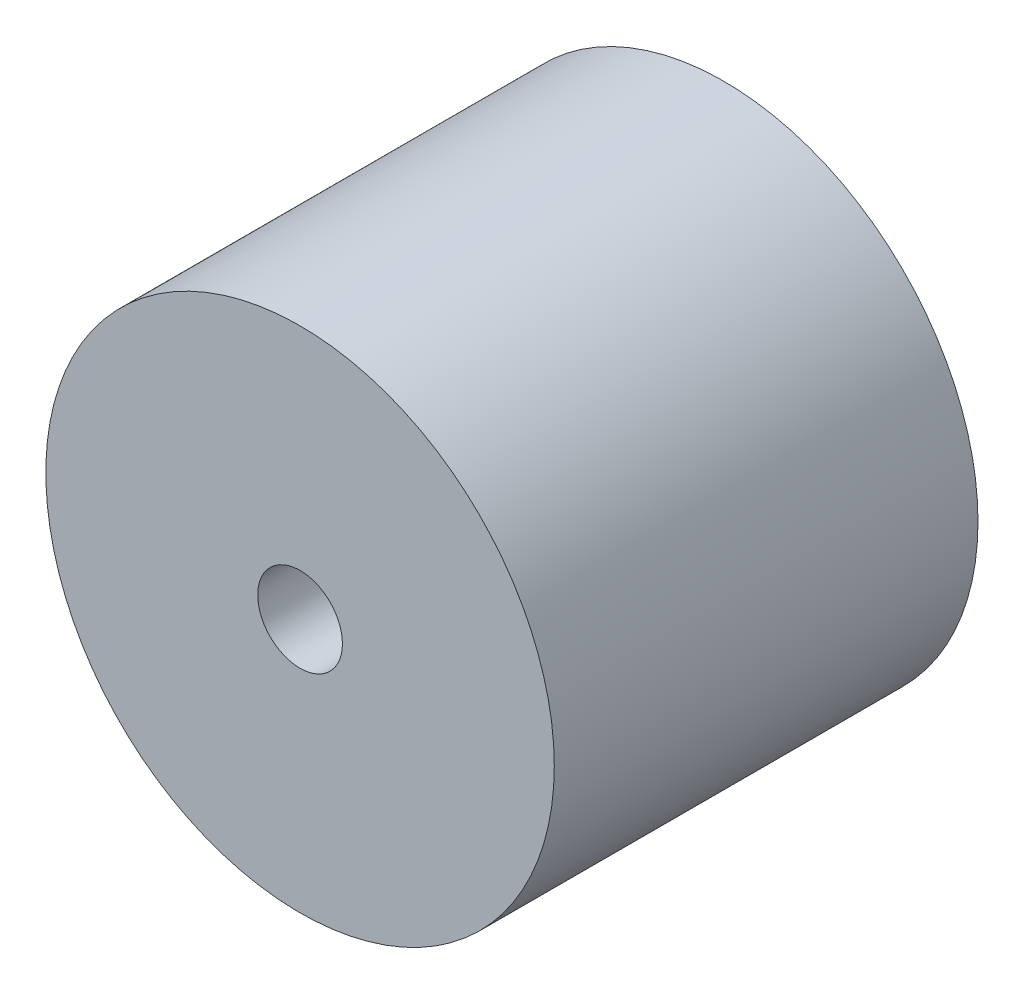
SolidWorks part; units mm, degrees
material "Plain Carbon Steel"
ref_plane "Front Plane" through (0, 0, 0) normal (0, 0, 1) x (1, 0, 0)
ref_plane "Top Plane" through (0, 0, 0) normal (0, 1, 0) x (1, 0, 0)
ref_plane "Right Plane" through (0, 0, 0) normal (1, 0, 0) x (0, 0, -1)
sketch "Bushing Profile Ø36-Ø6" plane through (0, 0, 0) normal (0, 0, 1) x (1, 0, 0)
  circle A0 centre (0, 0) radius 18
  circle A1 centre (0, 0) radius 3
  dimension "D1" = 36
  dimension "D2" = 6
extrude "Bushing Body L30" add sketch "Bushing Profile Ø36-Ø6" along normal mid plane 30
